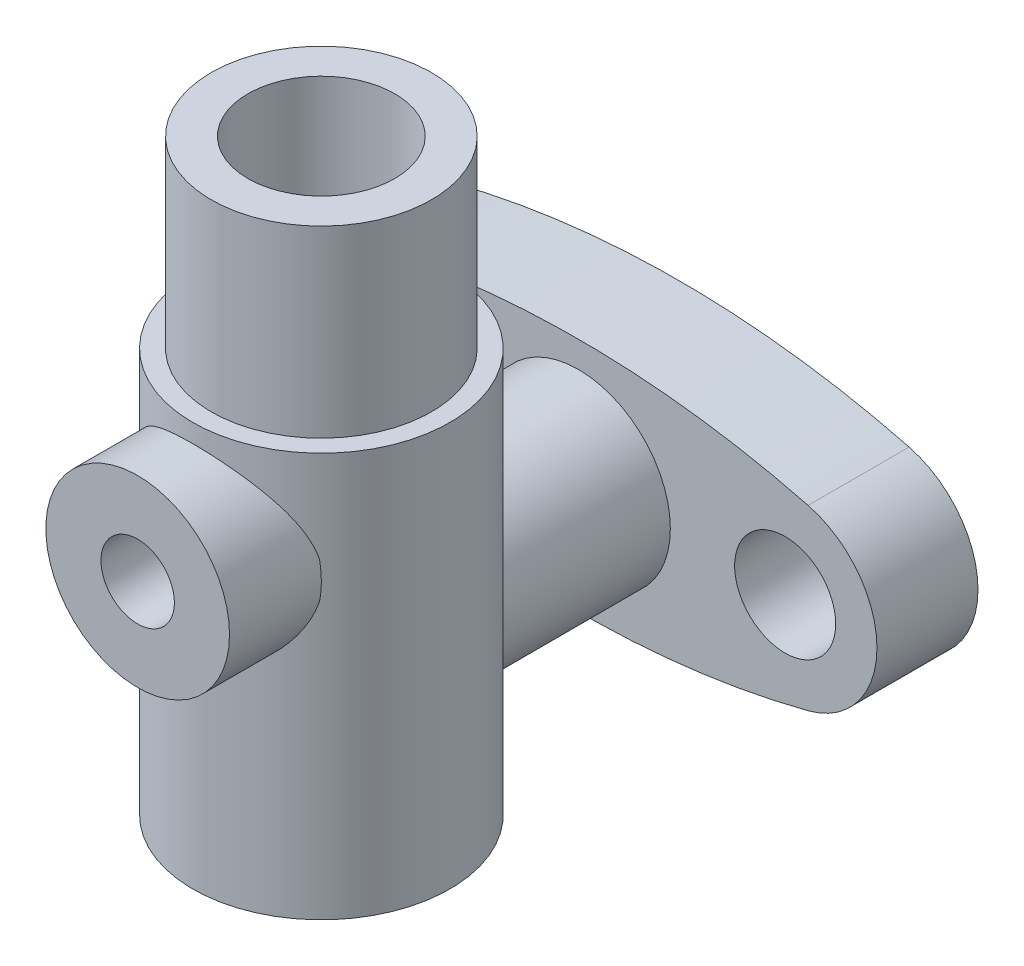
from build123d import *

# Parameters (mm, degrees)
SIDE_PORT_BOSS_SKETCH_R            = 10
SIDE_PORT_BOSS_DEPTH               = 10
MOUNTING_EAR_SKETCH_R              = 5.5
MOUNTING_EAR_DEPTH                 = 11
EAR_HUB_BOSS_REACH                 = 88.35
EAR_HUB_BOSS_END_RADIUS            = 14
EAR_HUB_SKETCH_R                   = 10
EAR_HOLE_8_D                       = 8
EAR_HOLE_8_DEPTH                   = 30
EAR_HOLE_8_TIP                     = 3.356398525
SIDE_PORT_TAPPED_HOLE_M8X1_0_D     = 8
SIDE_PORT_TAPPED_HOLE_M8X1_0_DEPTH = 17.596557524
SIDE_PORT_TAPPED_HOLE_M8X1_0_TIP   = 2.403442476


with BuildPart() as part:
    # Main Body Profile Sketch → Main Body Revolve (revolve)
    with BuildSketch(Plane.XY, mode=Mode.PRIVATE) as main_body_revolve_sk:
        Polygon((0, 64), (12, 64), (12, 44), (14, 44), (14, 0), (0, 0), align=None)
    revolve(main_body_revolve_sk.sketch.rotate(Axis((0, 64, 0), (0, -1, 0)), 180), axis=Axis((0, 64, 0), (0, -1, 0)))

    # Side Port Boss Sketch → Side Port Boss (add)
    with BuildSketch(Plane.XY.offset(20)):
        with Locations((0, 32)):
            Circle(SIDE_PORT_BOSS_SKETCH_R)
    extrude(amount=-SIDE_PORT_BOSS_DEPTH)



with BuildPart() as body_2:
    # Mounting Ear Sketch → Mounting Ear (new body)
    # profile 1 of 6: a face of its own
    with BuildSketch(Plane.XY.offset(-39)):
        with BuildLine():
            Line((0, 14), (0, 5.14212529))
            ThreePointArc((0, 5.14212529), (12.600429248, 5.939155663), (25, 8.317541634))
            ThreePointArc((25, 8.317541634), (32.5, 18), (25, 27.682458366))
            ThreePointArc((25, 27.682458366), (12.600429248, 30.060844337), (0, 30.85787471))
            Line((0, 30.85787471), (0, 22))
            ThreePointArc((0, 22), (2.828427125, 20.828427125), (4, 18))
            ThreePointArc((4, 18), (2.828427125, 15.171572875), (0, 14))
        make_face()
        with Locations((22.5, 18)):
            Circle(MOUNTING_EAR_SKETCH_R, mode=Mode.SUBTRACT)
    # profile 2 of 6: a face of its own
    with BuildSketch(Plane.XY.offset(-39)):
        with BuildLine():
            ThreePointArc((-25, 8.317541634), (-12.600429248, 5.939155663), (0, 5.14212529))
            Line((0, 5.14212529), (0, 14))
            ThreePointArc((0, 14), (-4, 18), (0, 22))
            Line((0, 22), (0, 30.85787471))
            ThreePointArc((0, 30.85787471), (-12.600429248, 30.060844337), (-25, 27.682458366))
            ThreePointArc((-25, 27.682458366), (-32.5, 18), (-25, 8.317541634))
        make_face()
        with Locations((-22.5, 18)):
            Circle(MOUNTING_EAR_SKETCH_R, mode=Mode.SUBTRACT)
    # profile 3 of 6: a face of its own
    with BuildSketch(Plane.XY.offset(-39)):
        with BuildLine():
            ThreePointArc((0, 22), (-4, 18), (0, 14))
            Line((0, 14), (0, 22))
        make_face()
    # profile 4 of 6: a face of its own
    with BuildSketch(Plane.XY.offset(-39)):
        with BuildLine():
            Line((0, 22), (0, 14))
            ThreePointArc((0, 14), (2.828427125, 15.171572875), (4, 18))
            ThreePointArc((4, 18), (2.828427125, 20.828427125), (0, 22))
        make_face()
    # profile 5 of 6: a face of its own
    with BuildSketch(Plane.XY.offset(-39)):
        with BuildLine():
            ThreePointArc((0, 22), (-4, 18), (0, 14))
            Line((0, 14), (0, 22))
        make_face()
    # profile 6 of 6: a face of its own
    with BuildSketch(Plane.XY.offset(-39)):
        with BuildLine():
            Line((0, 22), (0, 14))
            ThreePointArc((0, 14), (2.828427125, 15.171572875), (4, 18))
            ThreePointArc((4, 18), (2.828427125, 20.828427125), (0, 22))
        make_face()
    extrude(amount=MOUNTING_EAR_DEPTH)


with BuildPart() as part_1:
    add(part.part)

    add(body_2.part)  # Ear Hub Boss merges body 2
    # Ear Hub Boss: up to this cylinder (the profile starts outside it)
    ear_hub_boss_end = Plane(origin=(0, 18, 0), z_dir=(0, 1, 0)) * Cylinder(EAR_HUB_BOSS_END_RADIUS, 205.7, mode=Mode.PRIVATE)
    # Ear Hub Sketch → Ear Hub Boss (add, up to the surface)
    with BuildSketch(Plane.XY.offset(-28), mode=Mode.PRIVATE) as ear_hub_boss_sk1:
        with Locations(Location((0, 18, 0), (0, 0, 180))):
            Circle(EAR_HUB_SKETCH_R)
    ear_hub_boss_tool1 = extrude(ear_hub_boss_sk1.sketch, amount=EAR_HUB_BOSS_REACH, mode=Mode.PRIVATE) - ear_hub_boss_end
    add(ear_hub_boss_tool1.solids().sort_by_distance((0, 18, -28))[0])

    # Bore Profile Sketch → Bore Revolve Cut (revolve, cut)
    with BuildSketch(Plane(origin=(0, 0, 0), x_dir=(0, 0, -1), z_dir=(1, 0, 0)), mode=Mode.PRIVATE) as bore_revolve_cut_sk:
        Polygon((0, 64), (8, 64), (8, 49), (4, 46.690598923), (4, 33.732050808), (5, 32), (5, 28.92820323), (9, 22), (9, 12), (8, 12), (8, 0), (0, 0), align=None)
    revolve(bore_revolve_cut_sk.sketch.rotate(Axis((0, 64, 0), (0, -1, 0)), 180), axis=Axis((0, 64, 0), (0, -1, 0)), mode=Mode.SUBTRACT)

    # Ear Hole Ø8
    with Locations(Plane(origin=(0, 0, -39), x_dir=(-1, 0, 0), z_dir=(0, 0, -1))):
        with Locations((0, 18)):
            Hole(EAR_HOLE_8_D / 2, depth=EAR_HOLE_8_DEPTH)
            with Locations((0, 0, -(EAR_HOLE_8_DEPTH + EAR_HOLE_8_TIP / 2))):  # 100° drill point
                Cone(0, EAR_HOLE_8_D / 2, EAR_HOLE_8_TIP, mode=Mode.SUBTRACT)

    # Side Port Tapped Hole M8x1.0
    with Locations(Plane.XY.offset(20)):
        with Locations((0, 32)):
            Hole(SIDE_PORT_TAPPED_HOLE_M8X1_0_D / 2, depth=SIDE_PORT_TAPPED_HOLE_M8X1_0_DEPTH)
            with Locations((0, 0, -(SIDE_PORT_TAPPED_HOLE_M8X1_0_DEPTH + SIDE_PORT_TAPPED_HOLE_M8X1_0_TIP / 2))):  # 118° drill point
                Cone(0, SIDE_PORT_TAPPED_HOLE_M8X1_0_D / 2, SIDE_PORT_TAPPED_HOLE_M8X1_0_TIP, mode=Mode.SUBTRACT)


solid = part_1.part
